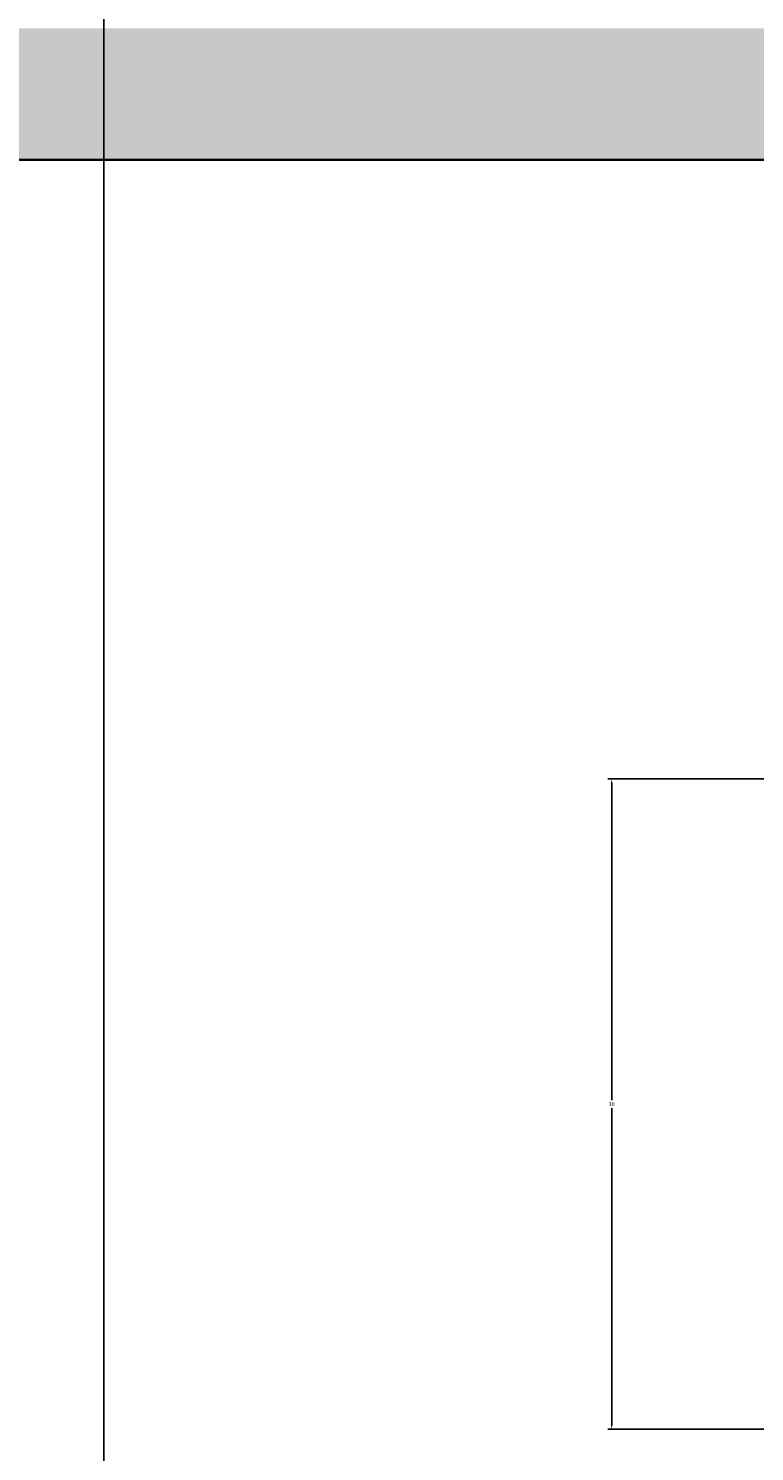
# Model space of a CAD drawing. Units: inches. Extents: x 2549 to 3108, y 1683 to 2362.
# Tile 8 of 30: x 2678 to 2711, y 2016 to 2081. Entities that reach past the tile are written whole.
import ezdxf

# ---------------------------------------------------------------- set-up
doc = ezdxf.new("R2010")
doc.units = ezdxf.units.IN
for name, color, linetype, lineweight in [('A-ANNO-DIMS', 2, 'Continuous', 18), ('A-WALL', 7, 'Continuous', 35), ('A-WALL-PATT', 89, 'Continuous', 13)]:
    doc.layers.add(name, color=color, linetype=linetype, lineweight=lineweight)
doc.layers.add('C-PKNG-VEHI-PATT', color=251, linetype='Continuous', lineweight=13, true_color=0x636466)
doc.layers.add('C-PVMT-PATT', color=9, linetype='Continuous', lineweight=13, true_color=0xc7c8ca)
doc.styles.get("Standard").update_dxf_attribs({"font": 'arial.ttf'})
doc.dimstyles.get("Standard").update_dxf_attribs({"dimtxt": 0.18, "dimasz": 0.18, "dimexe": 0.18, "dimexo": 0.0625, "dimgap": 0.09, "dimtad": 0, "dimtih": 1, "dimtoh": 1, "dimdec": 4, "dimzin": 0, "dimdsep": 46, "dimtxsty": 'Standard', "dimcen": 0.09, "dimadec": 0, "dimazin": 0, "dimtfac": 1, "dimtdec": 4, "dimtofl": 0, "dimtmove": 0, "dimatfit": 3, "dimfxl": 1, "dimtolj": 1, "dimtzin": 0, "dimarcsym": 0})

# ---------------------------------------------------------------- blocks, each defined once
blk = doc.blocks.new('*D21')
at = {"layer": 'A-ANNO-DIMS', "color": 0, "lineweight": -2, "transparency": 16777216}
for p, q in [((2711.452, 2046.283), (2703.972, 2046.283)), ((2704.152, 2046.103), (2704.152, 2031.633)), ((2704.152, 2016.798), (2704.152, 2031.269)), ((2711.452, 2016.618), (2703.972, 2016.618))]:
    blk.add_line(p, q, dxfattribs=at)
at = {"layer": 'A-ANNO-DIMS', "color": 0, "transparency": 16777216}
for points in [[(2704.122, 2046.103), (2704.182, 2046.103), (2704.152, 2046.283)], [(2704.122, 2016.798), (2704.182, 2016.798), (2704.152, 2016.618)]]:
    blk.add_solid(points, dxfattribs=at)
at = {"layer": 'Defpoints', "color": 0, "transparency": 16777216}
for p in [(2704.152, 2046.283), (2711.514, 2046.283), (2711.514, 2016.618)]:
    blk.add_point(p, dxfattribs=at)
at = {"layer": 'A-ANNO-DIMS', "color": 0, "transparency": 16777216, "insert": (2704.152, 2031.451), "char_height": 0.18, "attachment_point": 5}
blk.add_mtext('\\A1;30', dxfattribs=at)
blk = doc.blocks.new('*D42')
at = {"layer": 'A-ANNO-DIMS', "color": 0, "lineweight": -2, "transparency": 16777216}
for p, q in [((2638.643, 2080.461), (2638.643, 1683.444)), ((2728.643, 2080.461), (2728.643, 1683.444)), ((2638.823, 1683.624), (2683.424, 1683.624)), ((2728.463, 1683.624), (2683.861, 1683.624))]:
    blk.add_line(p, q, dxfattribs=at)
at = {"layer": 'A-ANNO-DIMS', "color": 0, "transparency": 16777216}
for points in [[(2638.823, 1683.654), (2638.823, 1683.594), (2638.643, 1683.624)], [(2728.463, 1683.654), (2728.463, 1683.594), (2728.643, 1683.624)]]:
    blk.add_solid(points, dxfattribs=at)
at = {"layer": 'Defpoints', "color": 0, "transparency": 16777216}
for p in [(2638.643, 2080.524), (2728.643, 2080.524), (2728.643, 1683.624)]:
    blk.add_point(p, dxfattribs=at)
at = {"layer": 'A-ANNO-DIMS', "color": 0, "transparency": 16777216, "insert": (2683.643, 1683.624), "char_height": 0.18, "attachment_point": 5}
blk.add_mtext('\\A1;90', dxfattribs=at)
blk = doc.blocks.new('*D44')
at = {"layer": 'A-ANNO-DIMS', "color": 0, "lineweight": -2, "transparency": 16777216}
for p, q in [((2662.643, 2040.993), (2662.643, 1683.444)), ((2806.643, 2016.129), (2806.643, 1683.444)), ((2662.823, 1683.624), (2734.363, 1683.624)), ((2806.463, 1683.624), (2734.923, 1683.624))]:
    blk.add_line(p, q, dxfattribs=at)
at = {"layer": 'A-ANNO-DIMS', "color": 0, "transparency": 16777216}
for points in [[(2662.823, 1683.654), (2662.823, 1683.594), (2662.643, 1683.624)], [(2806.463, 1683.654), (2806.463, 1683.594), (2806.643, 1683.624)]]:
    blk.add_solid(points, dxfattribs=at)
at = {"layer": 'Defpoints', "color": 0, "transparency": 16777216}
for p in [(2662.643, 2041.056), (2806.643, 2016.191), (2806.643, 1683.624)]:
    blk.add_point(p, dxfattribs=at)
at = {"layer": 'A-ANNO-DIMS', "color": 0, "transparency": 16777216, "insert": (2734.643, 1683.624), "char_height": 0.18, "attachment_point": 5}
blk.add_mtext('\\A1;144', dxfattribs=at)
blk = doc.blocks.new('*D59')
at = {"layer": 'A-ANNO-DIMS', "color": 0, "lineweight": -2, "transparency": 16777216}
for p, q in [((2680.978, 1761.586), (2680.978, 2362.323)), ((2681.158, 2362.143), (2733.112, 2362.143)), ((2785.978, 2362.143), (2734.023, 2362.143)), ((2786.158, 1761.586), (2786.158, 2362.323))]:
    blk.add_line(p, q, dxfattribs=at)
at = {"layer": 'A-ANNO-DIMS', "color": 0, "transparency": 16777216}
for points in [[(2681.158, 2362.173), (2681.158, 2362.113), (2680.978, 2362.143)], [(2785.978, 2362.173), (2785.978, 2362.113), (2786.158, 2362.143)]]:
    blk.add_solid(points, dxfattribs=at)
at = {"layer": 'Defpoints', "color": 0, "transparency": 16777216}
for p in [(2786.158, 2362.143), (2680.978, 1761.524), (2786.158, 1761.524)]:
    blk.add_point(p, dxfattribs=at)
at = {"layer": 'A-ANNO-DIMS', "color": 0, "transparency": 16777216, "insert": (2733.568, 2362.143), "char_height": 0.18, "attachment_point": 5}
blk.add_mtext('\\A1;105.18', dxfattribs=at)

msp = doc.modelspace()

# ---------------------------------------------------------------- hatches: boundary and pattern name
at = {"layer": 'A-WALL-PATT'}
h = msp.add_hatch(color=256, dxfattribs=at)
h.dxf.hatch_style = 1
h.paths.add_polyline_path([(2638.6427, 2272.5237), (3034.6427, 2272.5237), (3034.6427, 1936.5237), (3043.6427, 1936.5237), (3043.6427, 2281.5237), (2629.6427, 2281.5237), (2629.6427, 2074.5237), (2812.6427, 2074.5237), (2812.6427, 2140.5237), (2785.7177, 2140.5237), (2785.7177, 2134.5237), (2806.6427, 2134.5237), (2806.6427, 2080.5237), (2638.6427, 2080.5237)])
h.paths.add_polyline_path([(2638.6427, 1972.5237), (2662.6427, 1972.5237), (2662.6427, 2041.0557), (2653.6427, 2041.0557), (2653.6427, 1978.5237), (2629.6427, 1978.5237), (2629.6427, 1795.5237), (2662.6427, 1795.5237), (2881.6427, 1795.5237), (2881.6427, 1936.5237), (2965.9351, 1936.5237), (2965.9351, 1974.5439), (2959.9351, 1974.5439), (2959.9351, 1945.5237), (2881.6427, 1945.5237), (2872.6427, 1945.5237), (2872.6427, 1804.5237), (2662.6427, 1804.5237), (2638.6427, 1804.5237)])
at = {"layer": 'C-PKNG-VEHI-PATT'}
h = msp.add_hatch(color=256, dxfattribs=at)
h.dxf.hatch_style = 1
edge = h.paths.add_edge_path()
edge.add_ellipse((2935.7258, 1791.964), major_axis=(-50.66, 0), ratio=0.8423039, start_angle=248.165046, end_angle=265.722579)
edge.add_line((2938.911, 1834.5507), (2925.8653, 1834.5507))
edge.add_ellipse((2929.0505, 1791.964), major_axis=(50.66, 0), ratio=0.8423039, start_angle=94.277421, end_angle=111.834954)
edge.add_line((2912.8508, 1832.3947), (2914.2044, 1822.2495))
edge.add_ellipse((2930.6538, 1783.1023), major_axis=(-49.3014, 0), ratio=0.8423039, start_angle=-85.12993, end_angle=-67.208085, ccw=False)
edge.add_line((2927.1247, 1824.5225), (2937.6516, 1824.5225))
edge.add_ellipse((2934.1225, 1783.1023), major_axis=(49.3014, 0), ratio=0.8423039, start_angle=67.208085, end_angle=85.12993, ccw=False)
edge.add_line((2950.5719, 1822.2495), (2951.9255, 1832.3947))
edge = h.paths.add_edge_path()
edge.add_ellipse((2903.4793, 1857.3351), major_axis=(-34.7979, 0), ratio=0.8423039, start_angle=180, end_angle=209.43857)
edge.add_ellipse((2961.297, 1857.3351), major_axis=(34.7979, 0), ratio=0.8423039, start_angle=150.56143, end_angle=180)
edge.add_line((2926.4991, 1857.3351), (2926.4991, 1843.7609))
edge.add_ellipse((2924.1251, 1844.3143), major_axis=(-0.2209, 3.9278), ratio=0.6038336, start_angle=89.002014, end_angle=253.657408, ccw=False)
edge.add_line((2921.7512, 1844.2222), (2921.7512, 1853.3975))
edge.add_line((2921.7512, 1853.3975), (2925.269, 1855.8484))
edge.add_ellipse((2925.4782, 1855.4931), major_axis=(0.4584, 0), ratio=0.8423039, start_angle=90, end_angle=134.480211, ccw=False)
edge.add_line((2925.4782, 1855.8792), (2926.4991, 1855.8792))
edge.add_line((2926.4991, 1855.8792), (2926.4991, 1857.3351))
edge.add_ellipse((2961.297, 1857.3351), major_axis=(34.7979, 0), ratio=0.8423039, start_angle=150.56143, end_angle=180, ccw=False)
edge.add_line((2932.3882, 1873.6501), (2932.3882, 1875.7801))
edge.add_ellipse((2932.3882, 1875.3939), major_axis=(0.4584, 0), ratio=0.8423039, start_angle=90, end_angle=127.93313)
edge.add_line((2932.1366, 1875.7167), (2928.5915, 1873.7564))
edge.add_ellipse((2899.9271, 2002.4692), major_axis=(155.4756, 0), ratio=0.84230387, start_angle=-80.743434, end_angle=-77.445067, ccw=False)
edge.add_ellipse((2949.4402, 1715.2151), major_axis=(-189.1422, 0), ratio=0.84230387, start_angle=-79.790461, end_angle=-77.555373)
edge.add_ellipse((3300.3614, 1852.5642), major_axis=(-386.1662, 0), ratio=0.84230387, start_angle=-2.863715, end_angle=2.198541)
edge.add_ellipse((2929.0505, 1792.5159), major_axis=(-55.6192, 0), ratio=0.8423039, start_angle=-85.917589, end_angle=-72.280047, ccw=False)
edge.add_line((2925.7129, 1839.2798), (2939.0634, 1839.2798))
edge.add_ellipse((2935.7258, 1792.5159), major_axis=(55.6192, 0), ratio=0.8423039, start_angle=72.280047, end_angle=85.917589, ccw=False)
edge.add_ellipse((2564.4149, 1852.5642), major_axis=(-386.1662, 0), ratio=0.84230387, start_angle=177.801459, end_angle=182.863715)
edge.add_ellipse((2915.3361, 1715.2151), major_axis=(189.1422, 0), ratio=0.84230387, start_angle=77.555373, end_angle=79.790461)
edge.add_ellipse((2964.8492, 2002.4692), major_axis=(-155.4756, 0), ratio=0.84230387, start_angle=77.445067, end_angle=80.743434, ccw=False)
edge.add_line((2936.1848, 1873.7564), (2932.6397, 1875.7167))
edge.add_ellipse((2932.3882, 1875.3939), major_axis=(0.4584, 0), ratio=0.8423039, start_angle=52.06687, end_angle=90)
edge.add_line((2932.3882, 1875.7801), (2932.3882, 1873.6501))
edge.add_ellipse((2903.4793, 1857.3351), major_axis=(-34.7979, 0), ratio=0.8423039, start_angle=180, end_angle=209.43857, ccw=False)
edge.add_line((2938.2772, 1857.3351), (2938.2772, 1855.8792))
edge.add_line((2938.2772, 1855.8792), (2939.4059, 1855.8792))
edge.add_ellipse((2939.2981, 1855.4931), major_axis=(-0.4584, 0), ratio=0.8423039, start_angle=225.519789, end_angle=270, ccw=False)
edge.add_line((2939.5903, 1855.7906), (2943.0251, 1853.3975))
edge.add_line((2943.0251, 1853.3975), (2943.0251, 1844.2222))
edge.add_ellipse((2940.6512, 1844.3143), major_axis=(0.2209, 3.9278), ratio=0.6038336, start_angle=106.342592, end_angle=270.997986, ccw=False)
edge.add_line((2938.2772, 1843.7609), (2938.2772, 1857.3351))
edge = h.paths.add_edge_path()
edge.add_ellipse((2932.3882, 1865.1973), major_axis=(91.081, 0), ratio=0.8423039, start_angle=256.401865, end_angle=283.598135, ccw=False)
edge.add_line((2914.2044, 1790.0239), (2914.2044, 1778.3622))
edge.add_ellipse((2932.3882, 1853.5356), major_axis=(91.081, 0), ratio=0.8423039, start_angle=256.401865, end_angle=283.598135)
edge.add_line((2950.5719, 1778.3622), (2950.5719, 1790.0239))
edge = h.paths.add_edge_path()
edge.add_ellipse((2948.7383, 1772.3145), major_axis=(1.8336, 0), ratio=0.8423039, start_angle=0, end_angle=90)
edge.add_line((2948.7383, 1773.859), (2916.038, 1773.859))
edge.add_ellipse((2916.038, 1772.3145), major_axis=(1.8336, 0), ratio=0.8423039, start_angle=90, end_angle=180)
edge.add_line((2914.2044, 1772.3145), (2914.2044, 1760.2558))
edge.add_line((2914.2044, 1760.2558), (2950.5719, 1760.2558))
edge.add_line((2950.5719, 1760.2558), (2950.5719, 1772.3145))
h.paths.add_polyline_path([(2748.8496, 2101.6383), (2798.148, 2101.6383), (2798.148, 2111.4248), (2748.8496, 2111.4248)], flags=9)
h.paths.add_polyline_path([(2685.2081, 2101.489), (2719.3253, 2101.489), (2719.3253, 2111.2819), (2685.2081, 2111.2819)], flags=9)
h.paths.add_polyline_path([(2814.6852, 1907.1328), (2847.8384, 1907.1328), (2847.8384, 1916.9258), (2814.6852, 1916.9258)], flags=9)
h.paths.add_polyline_path([(2814.3906, 1835.5864), (2848.0172, 1835.5864), (2848.0172, 1845.3794), (2814.3906, 1845.3794)], flags=9)
h.paths.add_polyline_path([(2800.5245, 1759.1674), (2853.7435, 1759.1674), (2853.7435, 1768.954), (2800.5245, 1768.954)], flags=9)
h.paths.add_polyline_path([(2972.4611, 1807.3305), (3015.3943, 1807.3305), (3015.3943, 1817.117), (2972.4611, 1817.117)], flags=9)
h.paths.add_polyline_path([(2902.3327, 1888.6731), (2937.9131, 1888.6731), (2937.9131, 1898.4661), (2902.3327, 1898.4661)], flags=9)
h.paths.add_polyline_path([(2712.1779, 1878.9039), (2754.1257, 1878.9039), (2754.1257, 1888.6904), (2712.1779, 1888.6904)], flags=9)
h.paths.add_polyline_path([(2614.0056, 2012.812), (2650.0251, 2012.812), (2650.0251, 2022.4371), (2614.0056, 2022.4371)], flags=9)
h.paths.add_polyline_path([(2713.3129, 2003.1645), (2747.4237, 2003.1645), (2747.4237, 2012.951), (2713.3129, 2012.951)], flags=9)
h.paths.add_polyline_path([(2950.1379, 2001.6934), (2982.2992, 2001.6934), (2982.2992, 2011.48), (2950.1379, 2011.48)], flags=9)
h.paths.add_polyline_path([(2940.864, 2238.5537), (2997.5066, 2238.5537), (2997.5066, 2248.3466), (2940.864, 2248.3466)], flags=9)
h.paths.add_polyline_path([(2821.5457, 2202.8348), (2855.663, 2202.8348), (2855.663, 2212.6278), (2821.5457, 2212.6278)], flags=9)
h.paths.add_polyline_path([(2661.8026, 2238.6249), (2718.4451, 2238.6249), (2718.4451, 2248.4179), (2661.8026, 2248.4179)], flags=9)
at = {"layer": 'C-PVMT-PATT'}
h = msp.add_hatch(color=256, dxfattribs=at)
h.dxf.hatch_style = 1
h.paths.add_polyline_path([(3067.6427, 2305.5237), (2605.6427, 2305.5237), (2605.6427, 2074.5237), (2629.6427, 2074.5237), (2629.6427, 2281.5237), (3043.6427, 2281.5237), (3043.6427, 1885.5237), (3043.6427, 1872.8745), (3031.1672, 1872.8745), (3031.1672, 1862.5731), (2995.8054, 1862.5731), (2995.8054, 1872.8745), (2983.1752, 1872.8745), (2983.1752, 1885.5237), (2881.6427, 1885.5237), (2881.6427, 1795.5237), (2751.0977, 1795.5237), (2751.0977, 1761.5237), (2786.1577, 1761.5237), (2786.1577, 1723.5237), (2881.84, 1723.5237), (2881.84, 1714.5237), (3067.6427, 1714.5237), (3067.6427, 1723.5237)])
edge = h.paths.add_edge_path(flags=16)
edge.add_ellipse((2949.4402, 1710.9683), major_axis=(-194.1014, 0), ratio=0.84230387, start_angle=-77.874034, end_angle=-76.219471, ccw=False)
edge.add_ellipse((2949.4402, 1715.2151), major_axis=(-189.1422, 0), ratio=0.84230387, start_angle=-79.790461, end_angle=-77.555373, ccw=False)
edge.add_ellipse((2899.9271, 2002.4692), major_axis=(155.4756, 0), ratio=0.84230387, start_angle=-80.743434, end_angle=-77.445067)
edge.add_line((2928.5915, 1873.7564), (2932.3882, 1875.8558))
edge.add_line((2932.3882, 1875.8558), (2936.1848, 1873.7564))
edge.add_ellipse((2964.8492, 2002.4692), major_axis=(-155.4756, 0), ratio=0.84230387, start_angle=77.445067, end_angle=80.743434)
edge.add_ellipse((2915.3361, 1715.2151), major_axis=(189.1422, 0), ratio=0.84230387, start_angle=77.555373, end_angle=79.790461, ccw=False)
edge.add_ellipse((2915.3361, 1710.9683), major_axis=(-194.1014, 0), ratio=0.84230387, start_angle=256.219471, end_angle=257.874034, ccw=False)
edge.add_ellipse((2628.2871, 1850.2612), major_axis=(-327.2532, 0), ratio=0.84230387, start_angle=182.17995, end_angle=183.650428, ccw=False)
edge.add_ellipse((2955.5637, 1861.9334), major_axis=(-0.9168, 0), ratio=0.8423039, start_angle=180, end_angle=270, ccw=False)
edge.add_line((2956.4805, 1862.3857), (2956.4805, 1846.4866))
edge.add_ellipse((2955.5637, 1846.939), major_axis=(-0.9168, 0), ratio=0.8423039, start_angle=90, end_angle=180, ccw=False)
edge.add_ellipse((-3607.0606, 1835.832), major_axis=(-6562.6242, 0), ratio=0.84230387, start_angle=179.61613322, end_angle=180.09022909, ccw=False)
edge.add_ellipse((2955.5637, 1791.0926), major_axis=(0.9168, 0), ratio=0.8423039, start_angle=0, end_angle=90, ccw=False)
edge.add_line((2956.4805, 1791.545), (2956.4805, 1775.6459))
edge.add_ellipse((2955.5637, 1776.0982), major_axis=(0.9168, 0), ratio=0.8423039, start_angle=270, end_angle=360, ccw=False)
edge.add_ellipse((-3607.0606, 1835.832), major_axis=(-6562.6242, 0), ratio=0.84230387, start_angle=179.3813568, end_angle=179.47172853, ccw=False)
edge.add_ellipse((2954.5907, 1763.8768), major_axis=(-1.3752, 0), ratio=0.8423039, start_angle=179.371763, end_angle=248.464757, ccw=False)
edge.add_ellipse((-3607.519, 1835.832), major_axis=(-6564.0409, 0), ratio=0.842303863, start_angle=179.35344594, end_angle=179.37176282, ccw=False)
edge.add_ellipse((2952.6829, 1761.8002), major_axis=(3.2503, 0), ratio=0.8423039, start_angle=-90, end_angle=-0.646554, ccw=False)
edge.add_line((2952.6829, 1759.0625), (2912.0934, 1759.0625))
edge.add_ellipse((2912.0934, 1761.8002), major_axis=(3.2503, 0), ratio=0.8423039, start_angle=180.646554, end_angle=270, ccw=False)
edge.add_ellipse((9472.2953, 1835.832), major_axis=(-6564.0409, 0), ratio=0.842303871, start_angle=0.62823722, end_angle=0.6465541, ccw=False)
edge.add_ellipse((2910.1856, 1763.8768), major_axis=(1.3752, 0), ratio=0.8423039, start_angle=111.535244, end_angle=180.628237, ccw=False)
edge.add_ellipse((9471.8369, 1835.832), major_axis=(-6562.6242, 0), ratio=0.84230387, start_angle=0.52827147, end_angle=0.6465541, ccw=False)
edge.add_ellipse((2909.2126, 1776.0982), major_axis=(-0.9168, 0), ratio=0.8423039, start_angle=0, end_angle=90, ccw=False)
edge.add_line((2908.2958, 1775.6459), (2908.2958, 1791.545))
edge.add_ellipse((2909.2126, 1791.0926), major_axis=(-0.9168, 0), ratio=0.8423039, start_angle=-90, end_angle=0, ccw=False)
edge.add_ellipse((9471.8369, 1835.832), major_axis=(-6562.6242, 0), ratio=0.84230387, start_angle=-0.09022909, end_angle=0.38386678, ccw=False)
edge.add_ellipse((2909.2126, 1846.939), major_axis=(-0.9168, 0), ratio=0.8423039, start_angle=0, end_angle=90, ccw=False)
edge.add_line((2908.2958, 1846.4866), (2908.2958, 1862.3857))
edge.add_ellipse((2909.2126, 1861.9334), major_axis=(0.9168, 0), ratio=0.8423039, start_angle=90, end_angle=180, ccw=False)
edge.add_ellipse((3236.4892, 1850.2612), major_axis=(327.2532, 0), ratio=0.84230387, start_angle=176.349572, end_angle=177.82005, ccw=False)
edge = h.paths.add_edge_path(flags=0)
edge.add_ellipse((2903.4793, 1857.3351), major_axis=(-34.7979, 0), ratio=0.8423039, start_angle=180, end_angle=209.43857, ccw=False)
edge.add_line((2938.2772, 1857.3351), (2938.2772, 1855.8792))
edge.add_line((2938.2772, 1855.8792), (2939.4631, 1855.8792))
edge.add_line((2939.4631, 1855.8792), (2943.0251, 1853.3975))
edge.add_line((2943.0251, 1853.3975), (2943.0251, 1844.2222))
edge.add_ellipse((2940.6512, 1844.3143), major_axis=(0.2209, 3.9278), ratio=0.6038336, start_angle=106.342592, end_angle=270.997986, ccw=False)
edge.add_line((2938.2772, 1843.7609), (2938.2772, 1857.3351))
edge.add_ellipse((2903.4793, 1857.3351), major_axis=(-34.7979, 0), ratio=0.8423039, start_angle=180, end_angle=209.43857)
edge.add_ellipse((2961.297, 1857.3351), major_axis=(34.7979, 0), ratio=0.8423039, start_angle=150.56143, end_angle=180)
edge.add_line((2926.4991, 1857.3351), (2926.4991, 1843.7609))
edge.add_ellipse((2924.1251, 1844.3143), major_axis=(-0.2209, 3.9278), ratio=0.6038336, start_angle=89.002014, end_angle=253.657408, ccw=False)
edge.add_line((2921.7512, 1844.2222), (2921.7512, 1853.3975))
edge.add_line((2921.7512, 1853.3975), (2925.3132, 1855.8792))
edge.add_line((2925.3132, 1855.8792), (2926.4991, 1855.8792))
edge.add_line((2926.4991, 1855.8792), (2926.4991, 1857.3351))
edge.add_ellipse((2961.297, 1857.3351), major_axis=(34.7979, 0), ratio=0.8423039, start_angle=150.56143, end_angle=180, ccw=False)
edge = h.paths.add_edge_path(flags=0)
edge.add_ellipse((2929.0505, 1791.964), major_axis=(50.66, 0), ratio=0.8423039, start_angle=94.277421, end_angle=111.834954, ccw=False)
edge.add_line((2925.8653, 1834.5507), (2938.911, 1834.5507))
edge.add_ellipse((2935.7258, 1791.964), major_axis=(-50.66, 0), ratio=0.8423039, start_angle=248.165046, end_angle=265.722579, ccw=False)
edge.add_line((2951.9255, 1832.3947), (2950.5719, 1822.2495))
edge.add_ellipse((2934.1225, 1783.1023), major_axis=(49.3014, 0), ratio=0.8423039, start_angle=67.208085, end_angle=85.12993)
edge.add_line((2937.6516, 1824.5225), (2927.1247, 1824.5225))
edge.add_ellipse((2930.6538, 1783.1023), major_axis=(-49.3014, 0), ratio=0.8423039, start_angle=-85.12993, end_angle=-67.208085)
edge.add_line((2914.2044, 1822.2495), (2912.8508, 1832.3947))
edge = h.paths.add_edge_path(flags=0)
edge.add_line((2910.1338, 1829.4651), (2912.6432, 1821.2711))
edge.add_ellipse((5203.7787, 1816.4367), major_axis=(-2291.1426, 0), ratio=0.84230387, start_angle=-0.1208974, end_angle=0.3640763)
edge.add_line((2912.7012, 1801.8782), (2910.3305, 1792.5698))
edge.add_ellipse((9471.8369, 1835.832), major_axis=(-6561.7074, 0), ratio=0.84230387, start_angle=0.05559431, end_angle=0.37776419, ccw=False)
edge = h.paths.add_edge_path(flags=0)
edge.add_ellipse((-3607.0606, 1835.832), major_axis=(6561.7074, 0), ratio=0.84230387, start_angle=-0.37776419, end_angle=-0.05559431, ccw=False)
edge.add_line((2954.4458, 1792.5698), (2952.0751, 1801.8782))
edge.add_ellipse((660.9976, 1816.4367), major_axis=(2291.1426, 0), ratio=0.84230387, start_angle=-0.3640763, end_angle=0.1208974)
edge.add_line((2952.1331, 1821.2711), (2954.6425, 1829.4651))
edge = h.paths.add_edge_path(flags=0)
edge.add_ellipse((2932.3882, 1865.1973), major_axis=(91.081, 0), ratio=0.8423039, start_angle=256.401865, end_angle=283.598135)
edge.add_line((2950.5719, 1790.0239), (2950.5719, 1778.3622))
edge.add_ellipse((2932.3882, 1853.5356), major_axis=(91.081, 0), ratio=0.8423039, start_angle=256.401865, end_angle=283.598135, ccw=False)
edge.add_line((2914.2044, 1778.3622), (2914.2044, 1790.0239))
edge = h.paths.add_edge_path(flags=0)
edge.add_line((2916.038, 1773.859), (2948.7383, 1773.859))
edge.add_ellipse((2948.7383, 1772.3145), major_axis=(1.8336, 0), ratio=0.8423039, start_angle=0, end_angle=90, ccw=False)
edge.add_line((2950.5719, 1772.3145), (2950.5719, 1760.2558))
edge.add_line((2950.5719, 1760.2558), (2914.2044, 1760.2558))
edge.add_line((2914.2044, 1760.2558), (2914.2044, 1772.3145))
edge.add_ellipse((2916.038, 1772.3145), major_axis=(1.8336, 0), ratio=0.8423039, start_angle=90, end_angle=180, ccw=False)
h.paths.add_polyline_path([(2629.6427, 1978.5237), (2605.6427, 1978.5237), (2605.6427, 1723.5237), (2629.6427, 1723.5237), (2629.6427, 1795.5237)], flags=17)
h.paths.add_polyline_path([(2800.5245, 1759.1674), (2853.7435, 1759.1674), (2853.7435, 1768.954), (2800.5245, 1768.954)], flags=24)
h.paths.add_polyline_path([(2972.4611, 1807.3305), (3015.3943, 1807.3305), (3015.3943, 1817.117), (2972.4611, 1817.117)], flags=24)

# ---------------------------------------------------------------- linework, layer by layer
at = {"layer": 'A-WALL'}
msp.add_line((2629.6427, 2074.5237), (2812.6427, 2074.5237), dxfattribs=at)

# ---------------------------------------------------------------- dimensions: what is measured, and where the dimension line sits
at = {"layer": 'A-ANNO-DIMS'}
for base, p1, p2, override, picture, middle in [((2786.1577, 2362.1425), (2680.9778, 1761.5237), (2786.1577, 1761.5237), {"dimdec": 2, "dimlfac": 1, "dimrnd": 0, "dimzin": 0, "dimdsep": 46, "dimlunit": 2}, '*D59', (2733.5678, 2362.1425)), ((2728.6427, 1683.6237), (2638.6427, 2080.5237), (2728.6427, 2080.5237), {"dimdec": 0, "dimlfac": 1, "dimrnd": 0, "dimzin": 0, "dimdsep": 46, "dimlunit": 2}, '*D42', (2683.6427, 1683.6237)), ((2806.6427, 1683.6237), (2662.6427, 2041.0557), (2806.6427, 2016.1911), {"dimdec": 0, "dimlfac": 1, "dimrnd": 0, "dimzin": 0, "dimdsep": 46, "dimlunit": 2}, '*D44', (2734.6427, 1683.6237))]:
    dim = msp.add_linear_dim(base=base, p1=p1, p2=p2, dimstyle='Standard', override=override, dxfattribs=at)
    dim.commit()
    dim.dimension.update_dxf_attribs({"geometry": picture, "text_midpoint": middle})
dim = msp.add_linear_dim(base=(2704.1521, 2046.2834), p1=(2711.5145, 2016.6183), p2=(2711.5145, 2046.2834), angle=90, dimstyle='Standard', override={"dimdec": 0, "dimlfac": 1, "dimrnd": 0, "dimzin": 0, "dimdsep": 46, "dimlunit": 2}, dxfattribs=at)
dim.commit()
dim.dimension.update_dxf_attribs({"geometry": '*D21', "text_midpoint": (2704.1521, 2031.4509)})

doc.saveas('drawing.dxf')
